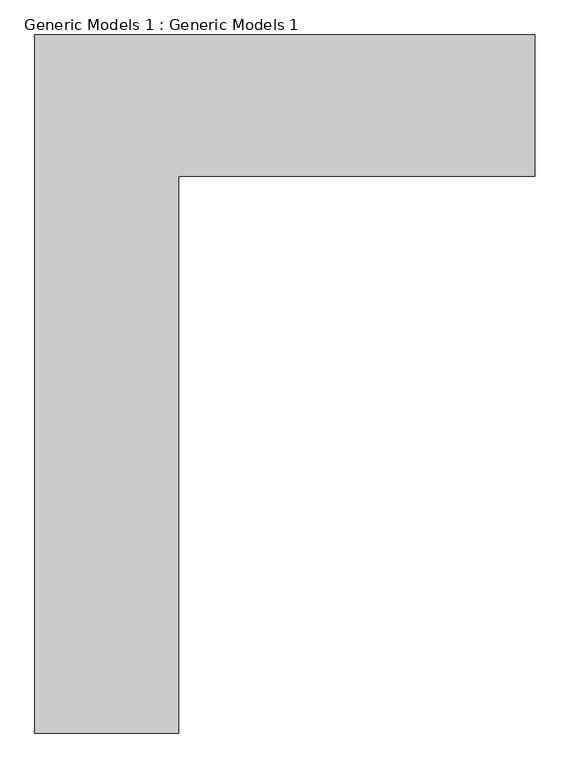
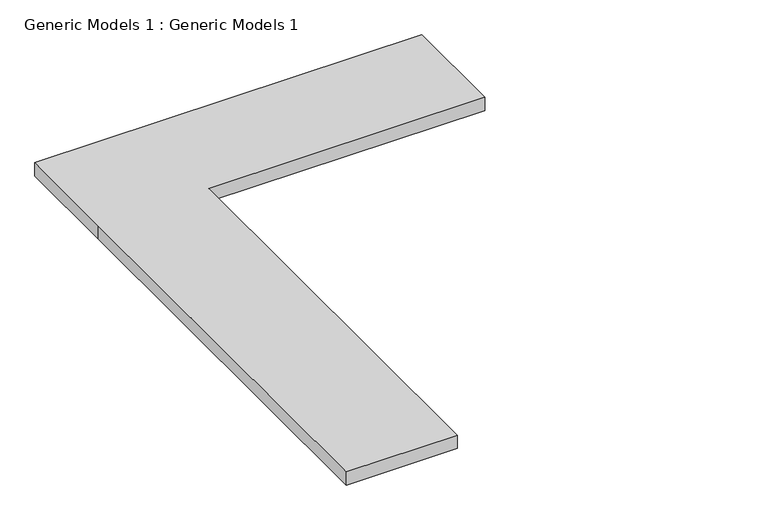
"""IFC4 building model written with IfcOpenShell, lengths in millimetres: proxy geometry, Generic Models 1 : Generic Models 1."""

from ifc_helpers import new_model, si_unit, frame, origin, place, context, project, spatial, polyline, outline, extrude, source, transform, mapped, element, save


def generic_models_1_generic_models_1_1574f5a2(model_context):
    return source(origin(), model_context, "Body", "SweptSolid", [
        extrude(outline(polyline([(-5258.2058888, 11253.510802), (-5258.2058888, 8899.3621562), (-5865.3374044, 8899.3621562), (-5865.3374044, 11253.510802), (-5865.3374044, 11850.4554997), (-3749.5174044, 11850.4554997), (-3749.5174044, 11253.510802), (-5258.2058888, 11253.510802)])), frame((0.0, 0.0, 1219.2), z_axis=(0.0, 0.0, 1.0), x_axis=(1.0, 0.0, 0.0)), (0.0, 0.0, 1.0), 76.2),
    ])


if __name__ == "__main__":
    model = new_model("IFC4")
    model_context = context("Model", 3, world=origin())
    ifc_project = project(units=[si_unit("LENGTHUNIT", "METRE", prefix="MILLI")], contexts=[model_context])
    site = spatial("IfcSite", under=ifc_project)
    building = spatial("IfcBuilding", under=site)
    placement = place(None, origin())
    generic_models_1_generic_models_1_shape = generic_models_1_generic_models_1_1574f5a2(model_context)
    element("IfcBuildingElementProxy", 1, Name="Generic Models 1 : Generic Models 1", ObjectType="Generic Models 1 : Generic Models 1", at=placement, inside=building, context=model_context, shape_type="MappedRepresentation", body=[
        mapped(generic_models_1_generic_models_1_shape, transform((0.0, 0.0, 0.0), x_axis=(1.0, 0.0, 0.0), y_axis=(0.0, 1.0, 0.0), z_axis=(0.0, 0.0, 1.0))),
    ])
    save(model, "model.ifc")

# Revit data of these elements
# Element 1 (IfcBuildingElementProxy, "Generic Models 1 : Generic Models 1")
#   Materials on its faces: "Concrete, Precast"
# Materials
#   "Concrete, Precast": class "Concrete", colour RGB 192 192 192, transparency 0, Description = "Precast concrete", Cost = 0
